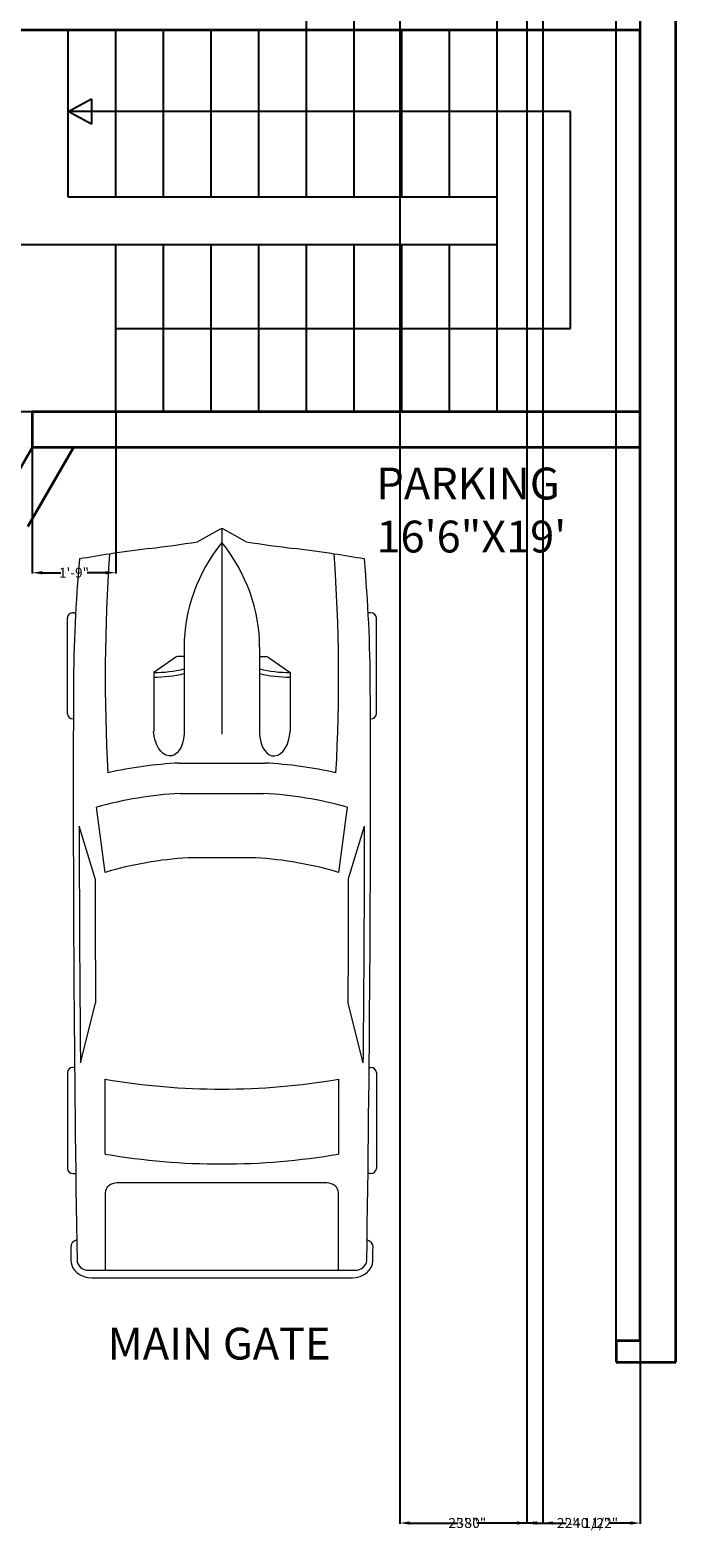
# Model space of a CAD drawing. Units: inches. Extents: x 1737 to 2270, y 2551 to 3419.
# Tile 2 of 4: x 2060 to 2222, y 2551 to 2930. Entities that reach past the tile are written whole.
import ezdxf

# ---------------------------------------------------------------- set-up
doc = ezdxf.new("R2010")
doc.units = ezdxf.units.IN
doc.header["$MEASUREMENT"] = 0
doc.layers.get('0').update_dxf_attribs({"color": 60})
for name, color, linetype, lineweight in [('A-ANNO-DIMS', 2, 'Continuous', 18), ('A-ANNO-TEXT', 231, 'Continuous', 18), ('A-AREA-IDEN', 231, 'Continuous', 18), ('EQUIPMENT', 7, 'Continuous', 13), ('STAIRCASE', 50, 'Continuous', 25), ('WALL', 60, 'Continuous', 35)]:
    doc.layers.add(name, color=color, linetype=linetype, lineweight=lineweight)
doc.styles.get("Standard").update_dxf_attribs({"font": 'arial.ttf'})
doc.dimstyles.get("Standard").update_dxf_attribs({"dimtxt": 2.5, "dimasz": 2.5, "dimexe": 0.18, "dimexo": 0.0625, "dimgap": 0.09, "dimtad": 0, "dimtih": 1, "dimtoh": 1, "dimzin": 0, "dimdsep": 46, "dimlunit": 3, "dimtxsty": 'Standard', "dimcen": 0.09, "dimadec": 0, "dimazin": 0, "dimtfac": 1, "dimtofl": 0, "dimtmove": 0, "dimatfit": 3, "dimfxl": 1, "dimtolj": 1, "dimtzin": 0, "dimarcsym": 0})

# ---------------------------------------------------------------- blocks, each defined once
blk = doc.blocks.new('*U4')
for p, q in [((46.55, 38.89), (22.35, 38.89)), ((136.7, 38.89), (160.9, 38.89)), ((21.1, 37.41), (21.1, 36.83)), ((47.8, 37.39), (47.8, 37.41)), ((87.99, 31.87), (74.76, 35.92)), ((134.31, 35.6), (119.29, 31.78)), ((135.45, 37.07), (135.45, 37.41)), ((162.15, 37.41), (162.15, 36.77)), ((70.03, 31.54), (86.41, 29.35)), ((186.47, -33.5), (186.47, 33.5)), ((188.4, -32.76), (188.4, 32.76)), ((138.42, 29.35), (157.25, 29.35)), ((186.47, 29.35), (167.01, 29.35)), ((164.52, 26.39), (164.52, -26.39)), ((32.27, 11.63), (36.13, 17.17)), ((36.13, 17.17), (50.94, 17.17)), ((29.77, 9.51), (51.68, 9.51)), ((32.12, 9.51), (32.12, 11.15)), ((58.92, -10.77), (58.92, 10.77)), ((66.55, -10.53), (66.55, 10.53)), ((82.74, 8.5), (82.74, -8.5)), ((186.47, -10.53), (186.47, 10.53)), ((3.27, 6.13), (0.1, 0.41)), ((0, 0), (51.68, 0)), ((0.1, -0.41), (3.27, -6.13)), ((29.77, -9.51), (51.68, -9.51)), ((32.12, -9.51), (32.12, -11.15)), ((32.27, -11.63), (36.13, -17.17)), ((36.13, -17.17), (50.94, -17.17)), ((86.41, -29.35), (70.03, -31.54)), ((157.25, -29.35), (138.42, -29.35)), ((167.01, -29.35), (186.47, -29.35)), ((87.99, -31.87), (74.76, -35.92)), ((134.31, -35.6), (119.29, -31.78)), ((21.1, -37.41), (21.1, -36.83)), ((47.8, -37.39), (47.8, -37.41)), ((135.45, -37.07), (135.45, -37.41)), ((162.15, -37.41), (162.15, -36.77)), ((46.55, -38.89), (22.35, -38.89)), ((136.7, -38.89), (160.9, -38.89))]:
    blk.add_line(p, q)
for centre, major_axis, ratio, start_param, end_param in [((22.35, 37.41), (0, -1.48), 0.842304, 3.141593, 4.712389), ((46.55, 37.41), (0, 1.48), 0.842304, -1.570796, 0), ((136.7, 37.41), (0, -1.48), 0.842304, 3.141593, 4.712389), ((160.9, 37.41), (0, 1.48), 0.842304, -1.570796, 0), ((180.63, 35.84), (0, 2.22), 0.842304, -0.013017, 1.249894), ((64.48, -10556.36), (0, 10595.31), 0.842304, -0.013397, -0.013017), ((183.98, 32.76), (0, -5.25), 0.842304, 1.570796, 3.128196), ((266.03, -27.52), (0, 313.31), 0.842304, 1.367076, 1.39176), ((41.19, -490.86), (0, 528.23), 0.842304, 0.00281, 0.075598), ((64.48, -10555.62), (0, 10593.03), 0.842304, -0.013397, 0.002797), ((64.48, -10555.62), (0, -10591.55), 0.842304, 3.133765, 3.140441), ((183.98, 33.5), (0, -2.96), 0.842304, 1.570796, 3.128196), ((135.29, 5.39), (0, 81.77), 0.842304, 1.245306, 1.50788), ((95.79, -3666.35), (0, -3698.24), 0.842304, 3.134049, 3.144098), ((259.18, -27.52), (0, -305.3), 0.842304, 4.528606, 4.561838), ((37.47, -593.96), (0, -623.33), 0.842304, 3.096046, 3.200911), ((134.4, 5.39), (0, -89.78), 0.842304, 4.449482, 4.652344), ((149.6, 2.8), (0, -79.58), 0.842304, 4.372215, 4.640744), ((17.08, 0), (0, 147.02), 0.842304, 4.511394, 4.913384), ((35.91, 0), (0, 147.02), 0.842304, 4.511394, 4.913384), ((167.01, 26.39), (0, 2.96), 0.842304, 0, 1.570796), ((-204.49, 52.4), (0, -250.96), 0.842304, 1.385369, 1.434372), ((13.04, 17.01), (0, 27.42), 0.842304, 4.435146, 4.718221), ((14.2, 17.01), (0, 27.42), 0.842304, 4.435146, 4.718221), ((50.79, 13.34), (6.34, -0.36), 0.603834, -1.395552, 1.581315), ((32.75, 11.15), (0, 0.74), 0.842304, 0.879714, 1.570796), ((29.77, -46.66), (0, 56.17), 0.842304, 0, 0.590319), ((0.62, 0), (0, -0.74), 0.842304, 4.131459, 5.293319), ((29.77, 46.66), (0, 56.17), 0.842304, 2.551274, 3.141593), ((-204.49, -52.4), (0, 250.96), 0.842304, -1.434372, -1.385369), ((32.75, -11.15), (0, -0.74), 0.842304, 4.712389, 5.403472), ((13.04, -17.01), (0, -27.42), 0.842304, 1.564964, 1.848039), ((14.2, -17.01), (0, -27.42), 0.842304, 1.564964, 1.848039), ((134.4, -5.39), (0, -89.78), 0.842304, -1.510751, -1.307889), ((135.29, -5.39), (0, -81.77), 0.842304, -1.50788, -1.245306), ((149.6, -2.8), (0, -79.58), 0.842304, -1.499151, -1.230623), ((259.18, 27.52), (0, 305.3), 0.842304, 1.721348, 1.754579), ((167.01, -26.39), (0, -2.96), 0.842304, 4.712389, 6.283185), ((266.03, 27.52), (0, 313.31), 0.842304, 1.749832, 1.774517), ((37.47, 593.96), (0, -623.33), 0.842304, -0.059319, 0.045547), ((95.79, 3666.35), (0, -3698.24), 0.842304, -0.002505, 0.007544), ((183.98, -33.5), (0, 2.96), 0.842304, 3.15499, 4.712389), ((183.98, -32.76), (0, -5.25), 0.842304, 0.013397, 1.570796), ((41.19, 490.86), (0, -528.23), 0.842304, -0.075598, -0.00281), ((22.35, -37.41), (0, 1.48), 0.842304, 1.570796, 3.141593), ((64.48, 10555.62), (0, 10593.03), 0.842304, 3.138796, 3.15499), ((46.55, -37.41), (0, -1.48), 0.842304, 0, 1.570796), ((64.48, 10555.62), (0, -10591.55), 0.842304, 0.001152, 0.007828), ((136.7, -37.41), (0, -1.48), 0.842304, -1.570796, 0), ((160.9, -37.41), (0, 1.48), 0.842304, 3.141593, 4.712389), ((180.63, -35.84), (0, -2.22), 0.842304, -1.249894, 0.013017), ((64.48, 10556.36), (0, 10595.31), 0.842304, 3.15461, 3.15499)]:
    blk.add_ellipse(centre, major_axis=major_axis, ratio=ratio, start_param=start_param, end_param=end_param)
at = {"extrusion": (0, 0, -1)}
blk.add_ellipse((50.79, -13.34), major_axis=(6.34, 0.36), ratio=0.603834, start_param=-1.395552, end_param=1.581315, dxfattribs=at)
blk = doc.blocks.new('*D20')
at = {"layer": 'A-ANNO-DIMS', "color": 0, "lineweight": -2, "transparency": 16777216}
for p, q in [((2022.87, 2595.22), (2022.87, 3415.79)), ((2025.37, 3415.61), (2107.86, 3415.61)), ((2204.71, 3415.61), (2122.22, 3415.61)), ((2207.21, 2595.22), (2207.21, 3415.79))]:
    blk.add_line(p, q, dxfattribs=at)
at = {"layer": 'A-ANNO-DIMS', "color": 0, "transparency": 16777216}
for points in [[(2025.37, 3416.02), (2025.37, 3415.19), (2022.87, 3415.61)], [(2204.71, 3416.02), (2204.71, 3415.19), (2207.21, 3415.61)]]:
    blk.add_solid(points, dxfattribs=at)
at = {"layer": 'Defpoints', "color": 0, "transparency": 16777216}
for p in [(2207.21, 3415.61), (2022.87, 2595.16), (2207.21, 2595.16)]:
    blk.add_point(p, dxfattribs=at)
at = {"layer": 'A-ANNO-DIMS', "color": 0, "transparency": 16777216, "insert": (2115.04, 3415.61), "char_height": 2.5, "attachment_point": 5}
blk.add_mtext('\\A1;15\'-4 1/2"', dxfattribs=at)
blk = doc.blocks.new('*D30')
at = {"layer": 'A-ANNO-DIMS', "color": 0, "lineweight": -2, "transparency": 16777216}
for p, q in [((2081.15, 2876.16), (2040.58, 2876.16)), ((2040.76, 2873.66), (2040.76, 2856.53)), ((2040.76, 2836.66), (2040.76, 2853.79)), ((2081.15, 2834.16), (2040.58, 2834.16))]:
    blk.add_line(p, q, dxfattribs=at)
at = {"layer": 'A-ANNO-DIMS', "color": 0, "transparency": 16777216}
for points in [[(2040.34, 2873.66), (2041.18, 2873.66), (2040.76, 2876.16)], [(2040.34, 2836.66), (2041.18, 2836.66), (2040.76, 2834.16)]]:
    blk.add_solid(points, dxfattribs=at)
at = {"layer": 'Defpoints', "color": 0, "transparency": 16777216}
for p in [(2040.76, 2876.16), (2081.21, 2876.16), (2081.21, 2834.16)]:
    blk.add_point(p, dxfattribs=at)
at = {"layer": 'A-ANNO-DIMS', "color": 0, "transparency": 16777216, "insert": (2040.76, 2855.16), "char_height": 2.5, "attachment_point": 5}
blk.add_mtext('\\A1;3\'-6"', dxfattribs=at)
blk = doc.blocks.new('*D31')
at = {"layer": 'A-ANNO-DIMS', "color": 0, "lineweight": -2, "transparency": 16777216}
for p, q in [((2129.21, 2930.22), (2129.21, 2970.79)), ((2131.71, 2970.61), (2131.91, 2970.61)), ((2138.71, 2970.61), (2138.5, 2970.61)), ((2141.21, 2930.22), (2141.21, 2970.79))]:
    blk.add_line(p, q, dxfattribs=at)
at = {"layer": 'A-ANNO-DIMS', "color": 0, "transparency": 16777216}
for points in [[(2131.71, 2971.02), (2131.71, 2970.19), (2129.21, 2970.61)], [(2138.71, 2971.02), (2138.71, 2970.19), (2141.21, 2970.61)]]:
    blk.add_solid(points, dxfattribs=at)
at = {"layer": 'Defpoints', "color": 0, "transparency": 16777216}
for p in [(2141.21, 2970.61), (2129.21, 2930.16), (2141.21, 2930.16)]:
    blk.add_point(p, dxfattribs=at)
at = {"layer": 'A-ANNO-DIMS', "color": 0, "transparency": 16777216, "insert": (2135.21, 2970.61), "char_height": 2.5, "attachment_point": 5}
blk.add_mtext('\\A1;1\'-0"', dxfattribs=at)
blk = doc.blocks.new('*D32')
at = {"layer": 'A-ANNO-DIMS', "color": 0, "lineweight": -2, "transparency": 16777216}
for p, q in [((2177.21, 2930.22), (2177.21, 2970.79)), ((2179.71, 2970.61), (2191.8, 2970.61)), ((2210.71, 2970.61), (2198.62, 2970.61)), ((2213.21, 2930.22), (2213.21, 2970.79))]:
    blk.add_line(p, q, dxfattribs=at)
at = {"layer": 'A-ANNO-DIMS', "color": 0, "transparency": 16777216}
for points in [[(2179.71, 2971.02), (2179.71, 2970.19), (2177.21, 2970.61)], [(2210.71, 2971.02), (2210.71, 2970.19), (2213.21, 2970.61)]]:
    blk.add_solid(points, dxfattribs=at)
at = {"layer": 'Defpoints', "color": 0, "transparency": 16777216}
for p in [(2213.21, 2970.61), (2177.21, 2930.16), (2213.21, 2930.16)]:
    blk.add_point(p, dxfattribs=at)
at = {"layer": 'A-ANNO-DIMS', "color": 0, "transparency": 16777216, "insert": (2195.21, 2970.61), "char_height": 2.5, "attachment_point": 5}
blk.add_mtext('\\A1;3\'-0"', dxfattribs=at)
blk = doc.blocks.new('*D35')
at = {"layer": 'A-ANNO-DIMS', "color": 0, "lineweight": -2, "transparency": 16777216}
for p, q in [((2152.71, 3066.6), (2152.71, 2554.53)), ((2188.71, 3066.6), (2188.71, 2554.53)), ((2155.21, 2554.71), (2167.3, 2554.71)), ((2186.21, 2554.71), (2174.12, 2554.71))]:
    blk.add_line(p, q, dxfattribs=at)
at = {"layer": 'A-ANNO-DIMS', "color": 0, "transparency": 16777216}
for points in [[(2155.21, 2555.12), (2155.21, 2554.29), (2152.71, 2554.71)], [(2186.21, 2555.12), (2186.21, 2554.29), (2188.71, 2554.71)]]:
    blk.add_solid(points, dxfattribs=at)
at = {"layer": 'Defpoints', "color": 0, "transparency": 16777216}
for p in [(2152.71, 3066.66), (2188.71, 3066.66), (2188.71, 2554.71)]:
    blk.add_point(p, dxfattribs=at)
at = {"layer": 'A-ANNO-DIMS', "color": 0, "transparency": 16777216, "insert": (2170.71, 2554.71), "char_height": 2.5, "attachment_point": 5}
blk.add_mtext('\\A1;3\'-0"', dxfattribs=at)
blk = doc.blocks.new('*D36')
at = {"layer": 'A-ANNO-DIMS', "color": 0, "lineweight": -2, "transparency": 16777216}
for p, q in [((2152.71, 3260.1), (2152.71, 2554.53)), ((2184.71, 3260.1), (2184.71, 2554.53)), ((2155.21, 2554.71), (2165.27, 2554.71)), ((2182.21, 2554.71), (2172.14, 2554.71))]:
    blk.add_line(p, q, dxfattribs=at)
at = {"layer": 'A-ANNO-DIMS', "color": 0, "transparency": 16777216}
for points in [[(2155.21, 2555.12), (2155.21, 2554.29), (2152.71, 2554.71)], [(2182.21, 2555.12), (2182.21, 2554.29), (2184.71, 2554.71)]]:
    blk.add_solid(points, dxfattribs=at)
at = {"layer": 'Defpoints', "color": 0, "transparency": 16777216}
for p in [(2152.71, 3260.16), (2184.71, 3260.16), (2184.71, 2554.71)]:
    blk.add_point(p, dxfattribs=at)
at = {"layer": 'A-ANNO-DIMS', "color": 0, "transparency": 16777216, "insert": (2168.71, 2554.71), "char_height": 2.5, "attachment_point": 5}
blk.add_mtext('\\A1;2\'-8"', dxfattribs=at)
blk = doc.blocks.new('*D42')
at = {"layer": 'A-ANNO-DIMS', "color": 0, "lineweight": -2, "transparency": 16777216}
for p, q in [((2184.71, 3263.5), (2184.71, 2554.53)), ((2213.21, 3264.1), (2213.21, 2554.53)), ((2187.21, 2554.71), (2192.61, 2554.71)), ((2210.71, 2554.71), (2205.31, 2554.71))]:
    blk.add_line(p, q, dxfattribs=at)
at = {"layer": 'A-ANNO-DIMS', "color": 0, "transparency": 16777216}
for points in [[(2187.21, 2555.12), (2187.21, 2554.29), (2184.71, 2554.71)], [(2210.71, 2555.12), (2210.71, 2554.29), (2213.21, 2554.71)]]:
    blk.add_solid(points, dxfattribs=at)
at = {"layer": 'Defpoints', "color": 0, "transparency": 16777216}
for p in [(2184.71, 3263.56), (2213.21, 3264.16), (2213.21, 2554.71)]:
    blk.add_point(p, dxfattribs=at)
at = {"layer": 'A-ANNO-DIMS', "color": 0, "transparency": 16777216, "insert": (2198.96, 2554.71), "char_height": 2.5, "attachment_point": 5}
blk.add_mtext('\\A1;2\'-4 1/2"', dxfattribs=at)
blk = doc.blocks.new('*D43')
at = {"layer": 'A-ANNO-DIMS', "color": 0, "lineweight": -2, "transparency": 16777216}
for p, q in [((2188.71, 3066.6), (2188.71, 2554.53)), ((2213.21, 3066.6), (2213.21, 2554.53)), ((2191.21, 2554.71), (2194.61, 2554.71)), ((2210.71, 2554.71), (2207.31, 2554.71))]:
    blk.add_line(p, q, dxfattribs=at)
at = {"layer": 'A-ANNO-DIMS', "color": 0, "transparency": 16777216}
for points in [[(2191.21, 2555.12), (2191.21, 2554.29), (2188.71, 2554.71)], [(2210.71, 2555.12), (2210.71, 2554.29), (2213.21, 2554.71)]]:
    blk.add_solid(points, dxfattribs=at)
at = {"layer": 'Defpoints', "color": 0, "transparency": 16777216}
for p in [(2188.71, 3066.66), (2213.21, 3066.66), (2213.21, 2554.71)]:
    blk.add_point(p, dxfattribs=at)
at = {"layer": 'A-ANNO-DIMS', "color": 0, "transparency": 16777216, "insert": (2200.96, 2554.71), "char_height": 2.5, "attachment_point": 5}
blk.add_mtext('\\A1;2\'-0 1/2"', dxfattribs=at)
blk = doc.blocks.new('*D46')
at = {"layer": 'A-ANNO-DIMS', "color": 0, "lineweight": -2, "transparency": 16777216}
for p, q in [((2060.21, 2834.1), (2060.21, 2793.53)), ((2081.21, 2834.1), (2081.21, 2793.53)), ((2062.71, 2793.71), (2067.41, 2793.71)), ((2078.71, 2793.71), (2074, 2793.71))]:
    blk.add_line(p, q, dxfattribs=at)
at = {"layer": 'A-ANNO-DIMS', "color": 0, "transparency": 16777216}
for points in [[(2062.71, 2794.12), (2062.71, 2793.29), (2060.21, 2793.71)], [(2078.71, 2794.12), (2078.71, 2793.29), (2081.21, 2793.71)]]:
    blk.add_solid(points, dxfattribs=at)
at = {"layer": 'Defpoints', "color": 0, "transparency": 16777216}
for p in [(2060.21, 2834.16), (2081.21, 2834.16), (2060.21, 2793.71)]:
    blk.add_point(p, dxfattribs=at)
at = {"layer": 'A-ANNO-DIMS', "color": 0, "transparency": 16777216, "insert": (2070.71, 2793.71), "char_height": 2.5, "attachment_point": 5}
blk.add_mtext('\\A1;1\'-9"', dxfattribs=at)

msp = doc.modelspace()

# ---------------------------------------------------------------- linework, layer by layer
at = {"layer": 'STAIRCASE'}
for p, q in [((2069.209, 2888.158), (2069.209, 2930.158)), ((2081.209, 2888.158), (2081.209, 2930.158)), ((2093.209, 2888.158), (2093.209, 2930.158)), ((2105.209, 2888.158), (2105.209, 2930.158)), ((2117.209, 2888.158), (2117.209, 2930.158)), ((2129.209, 2888.158), (2129.209, 2930.158)), ((2141.209, 2888.158), (2141.209, 2930.158)), ((2153.209, 2888.158), (2153.209, 2930.158)), ((2165.209, 2888.158), (2165.209, 2930.158)), ((2177.209, 2834.158), (2177.209, 2930.158)), ((2069.209, 2909.729), (2075.082, 2912.859)), ((2075.082, 2912.859), (2075.082, 2906.518)), ((2195.694, 2909.729), (2069.209, 2909.729)), ((2075.082, 2906.518), (2069.209, 2909.729)), ((2195.694, 2855.158), (2195.694, 2909.729)), ((2177.209, 2888.158), (2069.209, 2888.158)), ((2081.209, 2834.158), (2081.209, 2876.158)), ((2177.209, 2876.158), (2081.209, 2876.158)), ((2093.209, 2834.158), (2093.209, 2876.158)), ((2105.209, 2834.158), (2105.209, 2876.158)), ((2117.209, 2834.158), (2117.209, 2876.158)), ((2129.209, 2834.158), (2129.209, 2876.158)), ((2141.209, 2834.158), (2141.209, 2876.158)), ((2153.209, 2834.158), (2153.209, 2876.158)), ((2165.209, 2834.158), (2165.209, 2876.158)), ((2081.209, 2855.158), (2195.694, 2855.158))]:
    msp.add_line(p, q, dxfattribs=at)
at = {"layer": 'WALL'}
for p, q in [((2222.209, 2595.158), (2222.209, 3375.158)), ((2060.209, 2930.158), (2054.209, 2930.158)), ((2213.209, 2930.158), (2060.209, 2930.158)), ((2213.209, 2834.158), (2213.209, 2930.158)), ((2213.209, 2834.158), (2060.209, 2834.158)), ((2060.209, 2834.158), (2060.209, 2825.158)), ((2213.209, 2600.52), (2213.209, 2834.158)), ((2051.319, 2809.803), (2060.209, 2825.158)), ((2059.108, 2805.293), (2070.608, 2825.158)), ((2213.209, 2825.158), (2060.209, 2825.158)), ((2213.209, 2600.52), (2207.209, 2600.52)), ((2207.209, 2600.52), (2207.209, 2595.158)), ((2207.209, 2595.158), (2213.209, 2595.158)), ((2213.209, 2595.158), (2222.209, 2595.158))]:
    msp.add_line(p, q, dxfattribs=at)

# ---------------------------------------------------------------- block references
at = {"layer": 'EQUIPMENT', "rotation": 270}
msp.add_blockref('*U4', (2107.928, 2804.751), dxfattribs=at)

# ---------------------------------------------------------------- texts
at = {"layer": 'A-ANNO-TEXT', "insert": (2079.155, 2603.825), "char_height": 8, "attachment_point": 1}
msp.add_mtext_dynamic_manual_height_columns('MAIN GATE', width=60.91246, gutter_width=1, heights=[0], dxfattribs=at)
at = {"layer": 'A-AREA-IDEN', "insert": (2146.834, 2820.133), "char_height": 8, "attachment_point": 1}
msp.add_mtext_dynamic_manual_height_columns('PARKING\\P16\'6"X19\'', width=60.91246, gutter_width=1, heights=[0], dxfattribs=at)

# ---------------------------------------------------------------- dimensions: what is measured, and where the dimension line sits
at = {"layer": 'A-ANNO-DIMS'}
for base, p1, p2, picture, middle in [((2207.209, 3415.608), (2022.872, 2595.158), (2207.209, 2595.158), '*D20', (2115.041, 3415.608)), ((2213.209, 2554.708), (2184.709, 3263.558), (2213.209, 3264.158), '*D42', (2198.959, 2554.708)), ((2184.709, 2554.708), (2152.709, 3260.158), (2184.709, 3260.158), '*D36', (2168.709, 2554.708)), ((2188.709, 2554.708), (2152.709, 3066.658), (2188.709, 3066.658), '*D35', (2170.709, 2554.708)), ((2213.209, 2554.708), (2188.709, 3066.658), (2213.209, 3066.658), '*D43', (2200.959, 2554.708)), ((2141.209, 2970.608), (2129.209, 2930.158), (2141.209, 2930.158), '*D31', (2135.209, 2970.608)), ((2213.209, 2970.608), (2177.209, 2930.158), (2213.209, 2930.158), '*D32', (2195.209, 2970.608))]:
    dim = msp.add_linear_dim(base=base, p1=p1, p2=p2, dimstyle='Standard', override={"dimdec": 1, "dimlfac": 1, "dimrnd": 0, "dimzin": 1, "dimdsep": 46, "dimlunit": 4, "dimfrac": 2}, dxfattribs=at)
    dim.commit()
    dim.dimension.update_dxf_attribs({"geometry": picture, "text_midpoint": middle})
for base, p2, angle, picture, middle in [((2040.759, 2876.158), (2081.209, 2876.158), 90, '*D30', (2040.759, 2855.158)), ((2060.209, 2793.708), (2060.209, 2834.158), 180, '*D46', (2070.709, 2793.708))]:
    dim = msp.add_linear_dim(base=base, p1=(2081.209, 2834.158), p2=p2, angle=angle, dimstyle='Standard', override={"dimdec": 1, "dimlfac": 1, "dimrnd": 0, "dimzin": 1, "dimdsep": 46, "dimlunit": 4, "dimfrac": 2}, dxfattribs=at)
    dim.commit()
    dim.dimension.update_dxf_attribs({"geometry": picture, "text_midpoint": middle})

doc.saveas('drawing.dxf')
